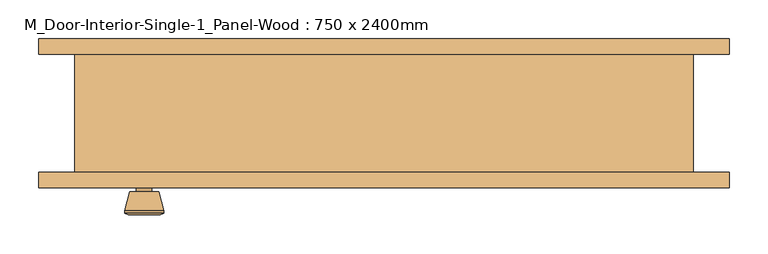
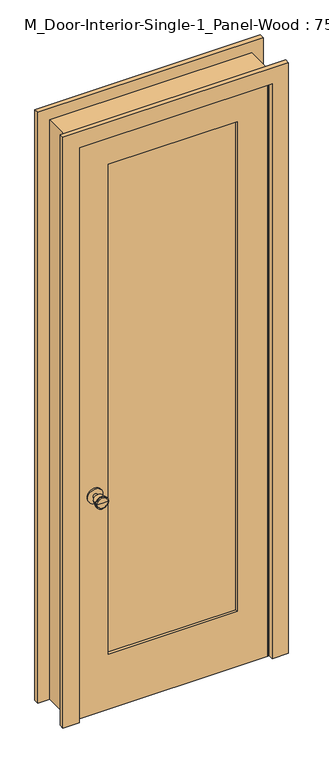
"""IFC4 building model written with IfcOpenShell, lengths in millimetres: door geometry, M_Door-Interior-Single-1_Panel-Wood : 750 x 2400mm."""

from ifc_helpers import new_model, si_unit, point, frame, frame_2d, origin, place, context, project, spatial, polyline, circle_curve, trimmed, segment, composite_curve, outline, extrude, faceted_brep, source, transform, mapped, element, save
from ifc_brep_helpers import plane_surface, cylinder_surface, revolved_surface, advanced_brep


def m_door_interior_single_1_panel_wood_750_x_2400mm_65023cff(model_context):
    return source(origin(), model_context, "Body", "SolidModel", [
        advanced_brep(
        [(-310.0, -32.025, 914.4), (-320.0, -32.025, 914.4), (-300.0, -32.025, 914.4), (-289.5241324, 16.975, 914.4), (-330.4758676, 16.975, 914.4), (-310.0, 16.975, 914.4), (-285.0, 15.1471319, 914.4), (-335.0, 15.1471319, 914.4), (-285.0, 11.6834537, 914.4), (-335.0, 11.6834537, 914.4), (-291.363764, -13.025, 914.4), (-328.636236, -13.025, 914.4), (-300.0, -13.025, 914.4), (-320.0, -13.025, 914.4)],
        [
            (0, 1),
            (1, 2, circle_curve(frame((-310.0, -32.025, 914.4), z_axis=(0.0, -1.0, 0.0), x_axis=(-1.0, 0.0, 0.0)), 10.0)),
            (2, 0),
            (2, 1, circle_curve(frame((-310.0, -32.025, 914.4), z_axis=(0.0, -1.0, 0.0), x_axis=(-1.0, 0.0, 0.0)), 10.0)),
            (3, 4, circle_curve(frame((-310.0, 16.975, 914.4), z_axis=(0.0, 1.0, 0.0), x_axis=(-1.0, 0.0, 0.0)), 20.4758676)),
            (4, 5),
            (5, 3),
            (4, 3, circle_curve(frame((-310.0, 16.975, 914.4), z_axis=(0.0, 1.0, 0.0), x_axis=(-1.0, 0.0, 0.0)), 20.4758676)),
            (6, 7, circle_curve(frame((-310.0, 15.1471319, 914.4), z_axis=(0.0, 1.0, 0.0), x_axis=(-1.0, 0.0, 0.0)), 25.0)),
            (7, 4),
            (3, 6),
            (7, 6, circle_curve(frame((-310.0, 15.1471319, 914.4), z_axis=(0.0, 1.0, 0.0), x_axis=(-1.0, 0.0, 0.0)), 25.0)),
            (8, 9, circle_curve(frame((-310.0, 11.6834537, 914.4), z_axis=(0.0, 1.0, 0.0), x_axis=(-1.0, 0.0, 0.0)), 25.0)),
            (9, 7),
            (6, 8),
            (9, 8, circle_curve(frame((-310.0, 11.6834537, 914.4), z_axis=(0.0, 1.0, 0.0), x_axis=(-1.0, 0.0, 0.0)), 25.0)),
            (10, 11, circle_curve(frame((-310.0, -13.025, 914.4), z_axis=(0.0, 1.0, 0.0), x_axis=(-1.0, 0.0, 0.0)), 18.636236)),
            (11, 9),
            (8, 10),
            (11, 10, circle_curve(frame((-310.0, -13.025, 914.4), z_axis=(0.0, 1.0, 0.0), x_axis=(-1.0, 0.0, 0.0)), 18.636236)),
            (12, 13, circle_curve(frame((-310.0, -13.025, 914.4), z_axis=(0.0, 1.0, 0.0), x_axis=(-1.0, 0.0, 0.0)), 10.0)),
            (13, 11),
            (10, 12),
            (13, 12, circle_curve(frame((-310.0, -13.025, 914.4), z_axis=(0.0, 1.0, 0.0), x_axis=(-1.0, 0.0, 0.0)), 10.0)),
            (1, 13),
            (12, 2),
        ],
        [
            plane_surface(frame((-310.0, -32.025, 914.4), z_axis=(0.0, -1.0, 0.0), x_axis=(-1.0, 0.0, 0.0))),
            plane_surface(frame((-310.0, 16.975, 914.4), z_axis=(0.0, 1.0, 0.0), x_axis=(-1.0, 0.0, 0.0))),
            revolved_surface(polyline([(-330.4758676, 16.975, 914.4), (-335.0, 15.1471319, 914.4)]), (-310.0, -32.025, 914.4), (0.0, -1.0, 0.0)),
            cylinder_surface(frame((-310.0, -32.025, 914.4), z_axis=(0.0, -1.0, 0.0), x_axis=(-1.0, 0.0, 0.0)), 25.0),
            revolved_surface(polyline([(-335.0, 11.6834537, 914.4), (-328.636236, -13.025, 914.4)]), (-310.0, -32.025, 914.4), (0.0, -1.0, 0.0)),
            plane_surface(frame((-310.0, -13.025, 914.4), z_axis=(0.0, -1.0, 0.0), x_axis=(-1.0, 0.0, 0.0))),
            cylinder_surface(frame((-310.0, -32.025, 914.4), z_axis=(0.0, -1.0, 0.0), x_axis=(-1.0, 0.0, 0.0)), 10.0),
        ],
        [
            (0, [[1, 2, 3]]),
            (0, [[-3, 4, -1]]),
            (1, [[5, 6, 7]]),
            (1, [[8, -7, -6]]),
            (2, [[9, 10, -5, 11]]),
            (2, [[12, -11, -8, -10]]),
            (3, [[13, 14, -9, 15]]),
            (3, [[16, -15, -12, -14]]),
            (4, [[17, 18, -13, 19]]),
            (4, [[20, -19, -16, -18]]),
            (5, [[21, 22, -17, 23]]),
            (5, [[24, -23, -20, -22]]),
            (6, [[-2, 25, -21, 26]]),
            (6, [[-4, -26, -24, -25]]),
        ],
    ),
        extrude(outline(composite_curve([segment(trimmed(circle_curve(frame_2d((914.4, -310.0)), 30.0), [point((914.4, -340.0))], [point((914.4, -280.0))], False, "CARTESIAN"), True, "CONTINUOUS"), segment(trimmed(circle_curve(frame_2d((914.4, -310.0)), 30.0), [point((914.4, -280.0))], [point((914.4, -340.0))], False, "CARTESIAN"), True, "CONTINUOUS")], self_intersect=False)), frame((0.0, -38.025, 0.0), z_axis=(0.0, 1.0, 0.0), x_axis=(0.0, 0.0, 1.0)), (0.0, 0.0, 1.0), 6.0),
        advanced_brep(
        [(-310.0, -79.025, 914.4), (-300.0, -79.025, 914.4), (-320.0, -79.025, 914.4), (-289.5241324, -128.025, 914.4), (-310.0, -128.025, 914.4), (-330.4758676, -128.025, 914.4), (-285.0, -126.1971319, 914.4), (-335.0, -126.1971319, 914.4), (-285.0, -122.7334537, 914.4), (-335.0, -122.7334537, 914.4), (-291.363764, -98.025, 914.4), (-328.636236, -98.025, 914.4), (-300.0, -98.025, 914.4), (-320.0, -98.025, 914.4)],
        [
            (0, 1),
            (1, 2, circle_curve(frame((-310.0, -79.025, 914.4), z_axis=(0.0, 1.0, 0.0), x_axis=(-1.0, 0.0, 0.0)), 10.0)),
            (2, 0),
            (2, 1, circle_curve(frame((-310.0, -79.025, 914.4), z_axis=(0.0, 1.0, 0.0), x_axis=(-1.0, 0.0, 0.0)), 10.0)),
            (3, 4),
            (4, 5),
            (5, 3, circle_curve(frame((-310.0, -128.025, 914.4), z_axis=(0.0, -1.0, 0.0), x_axis=(-1.0, 0.0, 0.0)), 20.4758676)),
            (3, 5, circle_curve(frame((-310.0, -128.025, 914.4), z_axis=(0.0, -1.0, 0.0), x_axis=(-1.0, 0.0, 0.0)), 20.4758676)),
            (6, 3),
            (5, 7),
            (7, 6, circle_curve(frame((-310.0, -126.1971319, 914.4), z_axis=(0.0, -1.0, 0.0), x_axis=(-1.0, 0.0, 0.0)), 25.0)),
            (6, 7, circle_curve(frame((-310.0, -126.1971319, 914.4), z_axis=(0.0, -1.0, 0.0), x_axis=(-1.0, 0.0, 0.0)), 25.0)),
            (8, 6),
            (7, 9),
            (9, 8, circle_curve(frame((-310.0, -122.7334537, 914.4), z_axis=(0.0, -1.0, 0.0), x_axis=(-1.0, 0.0, 0.0)), 25.0)),
            (8, 9, circle_curve(frame((-310.0, -122.7334537, 914.4), z_axis=(0.0, -1.0, 0.0), x_axis=(-1.0, 0.0, 0.0)), 25.0)),
            (10, 8),
            (9, 11),
            (11, 10, circle_curve(frame((-310.0, -98.025, 914.4), z_axis=(0.0, -1.0, 0.0), x_axis=(-1.0, 0.0, 0.0)), 18.636236)),
            (10, 11, circle_curve(frame((-310.0, -98.025, 914.4), z_axis=(0.0, -1.0, 0.0), x_axis=(-1.0, 0.0, 0.0)), 18.636236)),
            (12, 10),
            (11, 13),
            (13, 12, circle_curve(frame((-310.0, -98.025, 914.4), z_axis=(0.0, -1.0, 0.0), x_axis=(-1.0, 0.0, 0.0)), 10.0)),
            (12, 13, circle_curve(frame((-310.0, -98.025, 914.4), z_axis=(0.0, -1.0, 0.0), x_axis=(-1.0, 0.0, 0.0)), 10.0)),
            (1, 12),
            (13, 2),
        ],
        [
            plane_surface(frame((-310.0, -79.025, 914.4), z_axis=(0.0, 1.0, 0.0), x_axis=(-1.0, 0.0, 0.0))),
            plane_surface(frame((-310.0, -128.025, 914.4), z_axis=(0.0, -1.0, 0.0), x_axis=(-1.0, 0.0, 0.0))),
            revolved_surface(polyline([(-330.4758676, -128.025, 914.4), (-335.0, -126.1971319, 914.4)]), (-310.0, -79.025, 914.4), (0.0, 1.0, 0.0)),
            cylinder_surface(frame((-310.0, -79.025, 914.4), z_axis=(0.0, 1.0, 0.0), x_axis=(-1.0, 0.0, 0.0)), 25.0),
            revolved_surface(polyline([(-335.0, -122.7334537, 914.4), (-328.636236, -98.025, 914.4)]), (-310.0, -79.025, 914.4), (0.0, 1.0, 0.0)),
            plane_surface(frame((-310.0, -98.025, 914.4), z_axis=(0.0, 1.0, 0.0), x_axis=(-1.0, 0.0, 0.0))),
            cylinder_surface(frame((-310.0, -79.025, 914.4), z_axis=(0.0, 1.0, 0.0), x_axis=(-1.0, 0.0, 0.0)), 10.0),
        ],
        [
            (0, [[1, 2, 3]]),
            (0, [[-3, 4, -1]]),
            (1, [[5, 6, 7]]),
            (1, [[-6, -5, 8]]),
            (2, [[9, -7, 10, 11]]),
            (2, [[-10, -8, -9, 12]]),
            (3, [[13, -11, 14, 15]]),
            (3, [[-14, -12, -13, 16]]),
            (4, [[17, -15, 18, 19]]),
            (4, [[-18, -16, -17, 20]]),
            (5, [[21, -19, 22, 23]]),
            (5, [[-22, -20, -21, 24]]),
            (6, [[25, -23, 26, -2]]),
            (6, [[-26, -24, -25, -4]]),
        ],
    ),
        extrude(outline(composite_curve([segment(trimmed(circle_curve(frame_2d((914.4, -310.0)), 30.0), [point((914.4, -340.0))], [point((914.4, -280.0))], False, "CARTESIAN"), True, "CONTINUOUS"), segment(trimmed(circle_curve(frame_2d((914.4, -310.0)), 30.0), [point((914.4, -280.0))], [point((914.4, -340.0))], False, "CARTESIAN"), True, "CONTINUOUS")], self_intersect=False)), frame((0.0, -79.025, 0.0), z_axis=(0.0, 1.0, 0.0), x_axis=(0.0, 0.0, 1.0)), (0.0, 0.0, 1.0), 6.0),
        extrude(outline(polyline([(255.0, -49.6916667), (255.0, -61.3583333), (-255.0, -61.3583333), (-255.0, -49.6916667), (255.0, -49.6916667)])), frame((0.0, 0.0, 230.0), z_axis=(0.0, 0.0, 1.0), x_axis=(1.0, 0.0, 0.0)), (0.0, 0.0, 1.0), 2050.0),
        extrude(outline(polyline([(2400.0, -375.0), (0.0, -375.0), (0.0, 375.0), (2400.0, 375.0), (2400.0, -375.0)]), holes=[polyline([(2280.0, -255.0), (2280.0, 255.0), (230.0, 255.0), (230.0, -255.0), (2280.0, -255.0)])]), frame((0.0, -73.025, 0.0), z_axis=(0.0, 1.0, 0.0), x_axis=(0.0, 0.0, 1.0)), (0.0, 0.0, 1.0), 35.0),
        faceted_brep([(400.0, -73.025, 0.0), (375.0, -73.025, 0.0), (375.0, -38.025, 0.0), (362.3, -38.025, 0.0), (362.3, -3.1, 0.0), (375.0, -3.1, 0.0), (375.0, 79.375, 0.0), (400.0, 79.375, 0.0), (400.0, 79.375, 2425.0), (400.0, -73.025, 2425.0), (375.0, 79.375, 2400.0), (-375.0, 79.375, 2400.0), (-375.0, 79.375, 0.0), (-400.0, 79.375, 0.0), (-400.0, 79.375, 2425.0), (375.0, -3.1, 2400.0), (362.3, -3.1, 2387.3), (-362.3, -3.1, 2387.3), (-362.3, -3.1, 0.0), (-375.0, -3.1, 0.0), (-375.0, -3.1, 2400.0), (362.3, -38.025, 2387.3), (375.0, -38.025, 2400.0), (-375.0, -38.025, 2400.0), (-375.0, -38.025, 0.0), (-362.3, -38.025, 0.0), (-362.3, -38.025, 2387.3), (375.0, -73.025, 2400.0), (-400.0, -73.025, 2425.0), (-400.0, -73.025, 0.0), (-375.0, -73.025, 0.0), (-375.0, -73.025, 2400.0)], [[[0, 1, 2, 3, 4, 5, 6, 7]], [[7, 8, 9, 0]], [[6, 10, 11, 12, 13, 14, 8, 7]], [[5, 15, 10, 6]], [[4, 16, 17, 18, 19, 20, 15, 5]], [[3, 21, 16, 4]], [[2, 22, 23, 24, 25, 26, 21, 3]], [[1, 27, 22, 2]], [[0, 9, 28, 29, 30, 31, 27, 1]], [[8, 14, 28, 9]], [[15, 20, 11, 10]], [[21, 26, 17, 16]], [[27, 31, 23, 22]], [[29, 13, 12, 19, 18, 25, 24, 30]], [[14, 13, 29, 28]], [[20, 19, 12, 11]], [[26, 25, 18, 17]], [[31, 30, 24, 23]]]),
        extrude(outline(polyline([(0.0, 446.35), (2471.35, 446.35), (2471.35, -446.35), (0.0, -446.35), (0.0, -381.35), (2406.35, -381.35), (2406.35, 381.35), (0.0, 381.35), (0.0, 446.35)])), frame((0.0, 79.375, 0.0), z_axis=(0.0, 1.0, 0.0), x_axis=(0.0, 0.0, 1.0)), (0.0, 0.0, 1.0), 20.0),
        extrude(outline(polyline([(0.0, 446.35), (2471.35, 446.35), (2471.35, -446.35), (0.0, -446.35), (0.0, -381.35), (2406.35, -381.35), (2406.35, 381.35), (0.0, 381.35), (0.0, 446.35)])), frame((0.0, -93.025, 0.0), z_axis=(0.0, 1.0, 0.0), x_axis=(0.0, 0.0, 1.0)), (0.0, 0.0, 1.0), 20.0),
    ])


if __name__ == "__main__":
    model = new_model("IFC4")
    model_context = context("Model", 3, world=origin())
    ifc_project = project(units=[si_unit("LENGTHUNIT", "METRE", prefix="MILLI")], contexts=[model_context])
    site = spatial("IfcSite", under=ifc_project)
    building = spatial("IfcBuilding", under=site)
    placement = place(None, origin())
    m_door_interior_single_1_panel_wood_750_x_2400mm_shape = m_door_interior_single_1_panel_wood_750_x_2400mm_65023cff(model_context)
    element("IfcDoor", 1, ObjectType="M_Door-Interior-Single-1_Panel-Wood : 750 x 2400mm", at=placement, inside=building, context=model_context, shape_type="MappedRepresentation", body=[
        mapped(m_door_interior_single_1_panel_wood_750_x_2400mm_shape, transform((0.0, 0.0, 0.0), x_axis=(1.0, 0.0, 0.0), y_axis=(0.0, 1.0, 0.0), z_axis=(0.0, 0.0, 1.0))),
    ])
    save(model, "model.ifc")

# Revit data of these elements
# Type "M_Door-Interior-Single-1_Panel-Wood : 750 x 2400mm"
#   Type Mark = "8"
#   Assembly Code = "C1020300"
#   Analytic Construction = "Wooden"
#   Top Rail = 0' - 4.72441"
#   Thickness = 0' - 1.37795"
#   Thermal Resistance (R) = 2.5876 (h·ft²·°F)/BTU
#   Swing Angle [instance default] = 90.00°
#   Stiles = 0' - 4.72441"
#   Rough Width = 2' - 7.49606"
#   Rough Height = 7' - 11.47244"
#   Height = 7' - 10.48819"
#   Width = 2' - 5.52756"
#   Heat Transfer Coefficient (U) = 0.3865 BTU/(h·ft²·°F)
#   Bottom Rail = 0' - 9.05512"
#   Trim Material = Cherry
#   Panel Material = Cherry
#   Frame Material = Cherry
#   Door Handle Material = Aluminum
#   Visual Light Transmittance = 0
#   Solar Heat Gain Coefficient = 0
#   Wall Closure = (empty or 0)
#   Function = (empty or 0)
# Element 1 (IfcDoor, "M_Door-Interior-Single-1_Panel-Wood : 750 x 2400mm")
#   Materials on its faces: "Cherry", "Aluminum"
# Materials
#   "Cherry": class "Wood", colour RGB 226 177 128, transparency 0, Description = "Prunus Serotina", Cost = 0
#   "Aluminum": class "Metal", colour RGB 247 247 247, transparency 0, Description = "Aluminum 6061", Cost = 0
